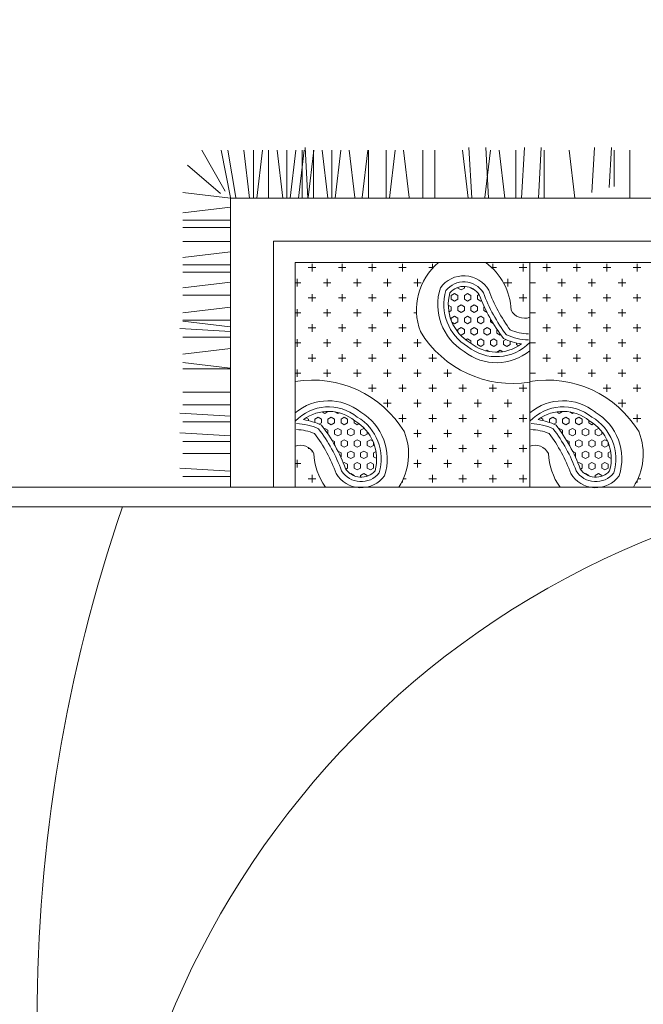
# Model space of a CAD drawing. Units: inches. Extents: x -638 to 186, y -762 to 59.
# Tile 8 of 31: x -140 to -118, y -492 to -457. Entities that reach past the tile are written whole.
import ezdxf

# ---------------------------------------------------------------- set-up
doc = ezdxf.new("R2010")
doc.units = ezdxf.units.IN
doc.layers.add('A-ANNO-DIMS', color=2, linetype='Continuous', lineweight=18)
doc.layers.add('furn', color=8, linetype='Continuous', lineweight=13)
doc.styles.get("Standard").update_dxf_attribs({"font": 'arial.ttf'})
doc.dimstyles.new('ISO-25', dxfattribs={"dimtxt": 4, "dimasz": 4, "dimexe": 1.25, "dimexo": 0.625, "dimtad": 0, "dimlunit": 4, "dimtxsty": 'Standard', "dimcen": 2.5, "dimclrt": 256, "dimadec": 0, "dimazin": 0, "dimtfac": 1, "dimtmove": 0, "dimatfit": 3, "dimfxl": 1, "dimfxlon": 1, "dimarcsym": 0})

# ---------------------------------------------------------------- blocks, each defined once
blk = doc.blocks.new('BED-DOUBLE-WITH-NIGHTSTANDS')
for p, q in [((58.548, 11.244), (58.548, 59.951)), ((57.828, 13.164), (57.828, 58.468)), ((58.923, 31.914), (58.923, 33.642)), ((59.126, 31.914), (59.228, 33.743)), ((59.755, 31.928), (59.755, 33.639)), ((60.193, 31.914), (60.193, 33.642)), ((60.397, 31.914), (60.499, 33.743)), ((60.906, 31.914), (60.906, 33.642)), ((61.11, 31.914), (61.212, 33.743)), ((61.517, 31.914), (61.517, 33.642)), ((61.977, 31.914), (61.977, 33.642)), ((62.81, 31.928), (62.81, 33.639)), ((62.841, 31.928), (63.044, 33.642)), ((63.554, 31.914), (63.35, 33.642)), ((63.961, 31.914), (63.961, 33.642)), ((64.165, 31.914), (64.266, 33.743)), ((64.327, 31.928), (64.531, 33.642)), ((64.572, 31.914), (64.572, 33.642)), ((65.04, 31.914), (64.836, 33.642)), ((65.476, 31.914), (65.476, 33.642)), ((65.944, 31.914), (65.741, 33.642)), ((66.309, 31.928), (66.309, 33.639)), ((66.573, 31.914), (66.573, 33.642)), ((67.041, 31.914), (66.838, 33.642)), ((67.406, 31.928), (67.406, 33.639)), ((67.922, 31.928), (67.922, 33.639)), ((68.186, 31.914), (68.186, 33.642)), ((68.654, 31.914), (68.45, 33.642)), ((68.982, 31.914), (69.186, 33.642)), ((69.142, 32.273), (70.169, 33.468)), ((69.232, 32.112), (70.71, 32.951)), ((68.996, 31.914), (70.707, 32.257)), ((68.996, 31.721), (70.707, 32.011)), ((58.548, 31.914), (68.982, 31.914)), ((68.982, 31.914), (68.982, 1.829)), ((68.982, 31.232), (70.71, 31.436)), ((68.982, 30.966), (70.71, 30.762)), ((68.996, 31.086), (70.707, 31.086)), ((58.548, 30.359), (67.427, 30.359)), ((67.427, 30.359), (67.427, 3.384)), ((68.982, 30.547), (70.71, 30.547)), ((68.982, 30.033), (70.71, 30.237)), ((68.996, 29.887), (70.707, 29.887)), ((58.548, 29.582), (66.65, 29.582)), ((59.258, 29.515), (59.53, 29.515)), ((59.394, 29.379), (59.394, 29.582)), ((62.523, 29.515), (62.795, 29.515)), ((62.659, 29.379), (62.659, 29.582)), ((63.612, 29.515), (63.884, 29.515)), ((63.748, 29.379), (63.748, 29.582)), ((64.7, 29.515), (64.972, 29.515)), ((64.836, 29.379), (64.836, 29.582)), ((65.788, 29.515), (66.06, 29.515)), ((65.924, 29.379), (65.924, 29.582)), ((66.65, 29.582), (66.65, 4.161)), ((68.982, 29.767), (70.71, 29.563)), ((61.047, 29.18), (61.003, 29.104)), ((68.982, 29.46), (70.71, 29.256)), ((68.982, 29.324), (70.71, 29.324)), ((68.982, 29.121), (70.811, 29.223)), ((58.714, 28.971), (58.986, 28.971)), ((58.85, 28.835), (58.85, 29.107)), ((59.802, 28.971), (59.857, 28.971)), ((59.938, 29.054), (59.938, 29.107)), ((61.003, 28.869), (60.881, 28.869)), ((61.003, 29.104), (60.948, 29.104)), ((61.003, 28.869), (61.072, 28.751)), ((63.067, 28.971), (63.339, 28.971)), ((63.203, 28.835), (63.203, 29.107)), ((64.156, 28.971), (64.428, 28.971)), ((64.292, 28.835), (64.292, 29.107)), ((65.244, 28.971), (65.516, 28.971)), ((65.38, 28.835), (65.38, 29.107)), ((66.332, 28.971), (66.605, 28.971)), ((66.468, 28.835), (66.468, 29.107)), ((68.982, 28.917), (70.71, 28.917)), ((68.996, 29.116), (70.71, 28.912)), ((60.663, 28.515), (60.595, 28.397)), ((60.652, 28.534), (60.663, 28.515)), ((60.821, 28.713), (60.867, 28.633)), ((61.003, 28.633), (60.867, 28.633)), ((61.072, 28.751), (61.003, 28.633)), ((61.261, 28.608), (61.208, 28.515)), ((61.208, 28.515), (61.276, 28.397)), ((62.659, 28.291), (62.659, 28.563)), ((63.748, 28.291), (63.748, 28.563)), ((64.836, 28.291), (64.836, 28.563)), ((65.924, 28.291), (65.924, 28.563)), ((68.982, 28.403), (70.71, 28.606)), ((60.187, 28.162), (60.075, 28.162)), ((60.245, 28.262), (60.187, 28.162)), ((60.459, 28.162), (60.391, 28.044)), ((60.459, 28.399), (60.459, 28.397)), ((60.595, 28.397), (60.459, 28.397)), ((60.595, 28.162), (60.459, 28.162)), ((60.595, 28.162), (60.663, 28.044)), ((60.867, 28.397), (60.799, 28.28)), ((60.799, 28.28), (60.867, 28.162)), ((61.003, 28.397), (60.867, 28.397)), ((61.003, 28.162), (60.867, 28.162)), ((61.003, 28.397), (61.072, 28.28)), ((61.072, 28.28), (61.003, 28.162)), ((61.258, 28.131), (61.208, 28.044)), ((61.279, 28.397), (61.276, 28.397)), ((62.523, 28.427), (62.795, 28.427)), ((63.612, 28.427), (63.884, 28.427)), ((64.7, 28.427), (64.972, 28.427)), ((65.788, 28.427), (66.06, 28.427)), ((68.982, 28.136), (70.71, 27.933)), ((68.996, 28.256), (70.707, 28.256)), ((59.199, 27.753), (59.235, 27.69)), ((59.439, 27.808), (59.371, 27.69)), ((59.419, 27.842), (59.439, 27.808)), ((59.637, 27.937), (59.643, 27.926)), ((59.779, 27.926), (59.643, 27.926)), ((59.843, 28.037), (59.779, 27.926)), ((60.051, 27.926), (59.983, 27.808)), ((59.983, 27.808), (60.051, 27.69)), ((60.187, 27.926), (60.051, 27.926)), ((60.187, 27.926), (60.255, 27.808)), ((60.255, 27.808), (60.187, 27.69)), ((60.391, 28.044), (60.459, 27.926)), ((60.595, 27.926), (60.459, 27.926)), ((60.663, 28.044), (60.595, 27.926)), ((60.867, 27.926), (60.799, 27.808)), ((60.799, 27.808), (60.867, 27.69)), ((61.003, 27.926), (60.867, 27.926)), ((61.003, 27.926), (61.072, 27.808)), ((61.072, 27.808), (61.003, 27.69)), ((61.208, 28.044), (61.231, 28.004)), ((63.067, 27.883), (63.339, 27.883)), ((63.203, 27.747), (63.203, 28.019)), ((64.156, 27.883), (64.428, 27.883)), ((64.292, 27.747), (64.292, 28.019)), ((65.244, 27.883), (65.516, 27.883)), ((65.38, 27.747), (65.38, 28.019)), ((66.332, 27.883), (66.605, 27.883)), ((66.468, 27.747), (66.468, 28.019)), ((58.963, 27.455), (58.955, 27.455)), ((59.031, 27.573), (58.963, 27.455)), ((59.025, 27.583), (59.031, 27.573)), ((59.235, 27.455), (59.167, 27.337)), ((59.371, 27.69), (59.235, 27.69)), ((59.371, 27.455), (59.235, 27.455)), ((59.371, 27.455), (59.439, 27.337)), ((59.643, 27.69), (59.575, 27.573)), ((59.575, 27.573), (59.643, 27.455)), ((59.779, 27.69), (59.643, 27.69)), ((59.779, 27.455), (59.643, 27.455)), ((59.779, 27.69), (59.847, 27.573)), ((59.847, 27.573), (59.779, 27.455)), ((60.051, 27.455), (59.983, 27.337)), ((60.187, 27.69), (60.051, 27.69)), ((60.187, 27.455), (60.051, 27.455)), ((60.187, 27.455), (60.255, 27.337)), ((60.459, 27.69), (60.391, 27.573)), ((60.391, 27.573), (60.459, 27.455)), ((60.595, 27.69), (60.459, 27.69)), ((60.595, 27.455), (60.459, 27.455)), ((60.595, 27.69), (60.663, 27.573)), ((60.663, 27.573), (60.595, 27.455)), ((60.867, 27.455), (60.799, 27.337)), ((61.003, 27.69), (60.867, 27.69)), ((60.958, 27.455), (60.867, 27.455)), ((62.659, 27.203), (62.659, 27.475)), ((63.748, 27.203), (63.748, 27.475)), ((64.836, 27.203), (64.836, 27.475)), ((65.924, 27.203), (65.924, 27.475)), ((68.996, 27.424), (70.71, 27.627)), ((58.963, 27.219), (58.904, 27.219)), ((58.963, 27.219), (59.031, 27.101)), ((59.031, 27.101), (58.963, 26.984)), ((59.167, 27.337), (59.235, 27.219)), ((59.371, 27.219), (59.235, 27.219)), ((59.439, 27.337), (59.371, 27.219)), ((59.643, 27.219), (59.575, 27.101)), ((59.575, 27.101), (59.643, 26.984)), ((59.779, 27.219), (59.643, 27.219)), ((59.779, 27.219), (59.847, 27.101)), ((59.847, 27.101), (59.779, 26.984)), ((59.983, 27.337), (60.051, 27.219)), ((60.187, 27.219), (60.051, 27.219)), ((60.255, 27.337), (60.187, 27.219)), ((60.459, 27.219), (60.391, 27.101)), ((60.391, 27.101), (60.459, 26.984)), ((60.595, 27.219), (60.459, 27.219)), ((60.595, 27.219), (60.663, 27.101)), ((60.663, 27.101), (60.637, 27.055)), ((60.799, 27.337), (60.836, 27.274)), ((62.523, 27.339), (62.795, 27.339)), ((63.612, 27.339), (63.884, 27.339)), ((64.7, 27.339), (64.972, 27.339)), ((65.788, 27.339), (66.06, 27.339)), ((68.996, 27.156), (70.71, 26.953)), ((58.963, 26.984), (58.94, 26.984)), ((59.235, 26.984), (59.167, 26.866)), ((59.167, 26.866), (59.235, 26.748)), ((59.371, 26.984), (59.235, 26.984)), ((59.371, 26.748), (59.235, 26.748)), ((59.371, 26.984), (59.439, 26.866)), ((59.439, 26.866), (59.371, 26.748)), ((59.643, 26.748), (59.58, 26.638)), ((59.779, 26.984), (59.643, 26.984)), ((59.779, 26.748), (59.643, 26.748)), ((59.779, 26.748), (59.83, 26.661)), ((60.051, 26.984), (59.983, 26.866)), ((59.983, 26.866), (60.051, 26.748)), ((60.187, 26.984), (60.051, 26.984)), ((60.144, 26.748), (60.051, 26.748)), ((60.187, 26.984), (60.255, 26.866)), ((60.255, 26.866), (60.201, 26.772)), ((60.553, 26.984), (60.459, 26.984)), ((61.979, 26.795), (62.251, 26.795)), ((62.115, 26.659), (62.115, 26.931)), ((63.067, 26.795), (63.339, 26.795)), ((63.203, 26.659), (63.203, 26.931)), ((64.156, 26.795), (64.428, 26.795)), ((64.292, 26.659), (64.292, 26.931)), ((65.244, 26.795), (65.516, 26.795)), ((65.38, 26.659), (65.38, 26.931)), ((66.332, 26.795), (66.605, 26.795)), ((66.468, 26.659), (66.468, 26.931)), ((68.996, 26.933), (70.707, 26.933)), ((61.571, 26.114), (61.571, 26.386)), ((62.659, 26.114), (62.659, 26.386)), ((63.748, 26.114), (63.748, 26.386)), ((64.836, 26.114), (64.836, 26.386)), ((65.924, 26.114), (65.924, 26.386)), ((61.435, 26.25), (61.707, 26.25)), ((62.523, 26.25), (62.795, 26.25)), ((63.612, 26.25), (63.884, 26.25)), ((64.7, 26.25), (64.972, 26.25)), ((65.788, 26.25), (66.06, 26.25)), ((68.982, 26.177), (70.71, 25.974)), ((68.996, 26.297), (70.707, 26.297)), ((58.714, 25.706), (58.783, 25.706)), ((58.85, 25.57), (58.85, 25.675)), ((60.891, 25.706), (61.163, 25.706)), ((61.027, 25.57), (61.027, 25.842)), ((61.979, 25.706), (62.251, 25.706)), ((62.115, 25.57), (62.115, 25.842)), ((63.067, 25.706), (63.339, 25.706)), ((63.203, 25.57), (63.203, 25.842)), ((64.156, 25.706), (64.428, 25.706)), ((64.292, 25.57), (64.292, 25.842)), ((65.244, 25.706), (65.516, 25.706)), ((65.38, 25.57), (65.38, 25.842)), ((66.332, 25.706), (66.605, 25.706)), ((66.468, 25.57), (66.468, 25.842)), ((68.996, 25.465), (70.71, 25.668)), ((59.394, 25.026), (59.394, 25.298)), ((60.483, 25.026), (60.483, 25.298)), ((61.571, 25.026), (61.571, 25.298)), ((62.659, 25.026), (62.659, 25.298)), ((63.748, 25.026), (63.748, 25.298)), ((64.836, 25.2), (64.836, 25.298)), ((65.924, 25.026), (65.924, 25.298)), ((59.258, 25.162), (59.53, 25.162)), ((60.346, 25.162), (60.619, 25.162)), ((61.435, 25.162), (61.707, 25.162)), ((62.523, 25.162), (62.795, 25.162)), ((63.612, 25.162), (63.884, 25.162)), ((65.788, 25.162), (66.06, 25.162)), ((68.996, 24.973), (70.707, 24.973)), ((58.714, 24.618), (58.986, 24.618)), ((58.85, 24.482), (58.85, 24.754)), ((59.802, 24.618), (60.074, 24.618)), ((59.938, 24.482), (59.938, 24.754)), ((60.891, 24.618), (61.163, 24.618)), ((61.027, 24.482), (61.027, 24.754)), ((61.979, 24.618), (62.251, 24.618)), ((62.115, 24.482), (62.115, 24.754)), ((63.067, 24.618), (63.339, 24.618)), ((63.203, 24.482), (63.203, 24.754)), ((66.45, 24.618), (66.605, 24.618)), ((66.468, 24.601), (66.468, 24.754)), ((68.996, 24.543), (70.707, 24.543)), ((59.394, 23.938), (59.394, 24.21)), ((60.483, 23.938), (60.483, 24.21)), ((61.571, 23.938), (61.571, 24.21)), ((62.659, 23.938), (62.659, 24.21)), ((59.258, 24.074), (59.53, 24.074)), ((60.346, 24.074), (60.619, 24.074)), ((61.435, 24.074), (61.707, 24.074)), ((62.523, 24.074), (62.795, 24.074)), ((64.44, 23.825), (64.495, 23.919)), ((64.508, 23.707), (64.44, 23.825)), ((64.552, 23.942), (64.644, 23.942)), ((64.712, 23.825), (64.644, 23.942)), ((64.644, 23.707), (64.712, 23.825)), ((64.917, 23.942), (64.866, 24.03)), ((64.917, 23.942), (65.053, 23.942)), ((65.053, 23.942), (65.116, 24.052)), ((65.257, 23.825), (65.325, 23.942)), ((65.325, 23.707), (65.257, 23.825)), ((65.325, 23.942), (65.461, 23.942)), ((65.529, 23.825), (65.461, 23.942)), ((65.461, 23.707), (65.529, 23.825)), ((58.714, 23.53), (58.986, 23.53)), ((58.85, 23.393), (58.85, 23.666)), ((59.802, 23.53), (60.074, 23.53)), ((59.938, 23.393), (59.938, 23.666)), ((60.891, 23.53), (61.163, 23.53)), ((61.027, 23.393), (61.027, 23.666)), ((61.979, 23.53), (62.251, 23.53)), ((62.115, 23.393), (62.115, 23.666)), ((64.032, 23.589), (64.059, 23.635)), ((64.1, 23.471), (64.032, 23.589)), ((64.1, 23.471), (64.236, 23.471)), ((64.143, 23.707), (64.236, 23.707)), ((64.304, 23.589), (64.236, 23.707)), ((64.236, 23.471), (64.304, 23.589)), ((64.44, 23.353), (64.508, 23.471)), ((64.508, 23.707), (64.644, 23.707)), ((64.508, 23.471), (64.644, 23.471)), ((64.712, 23.353), (64.644, 23.471)), ((64.849, 23.589), (64.917, 23.707)), ((64.917, 23.471), (64.849, 23.589)), ((64.917, 23.707), (65.053, 23.707)), ((64.917, 23.471), (65.053, 23.471)), ((65.121, 23.589), (65.053, 23.707)), ((65.053, 23.471), (65.121, 23.589)), ((65.257, 23.353), (65.325, 23.471)), ((65.325, 23.707), (65.461, 23.707)), ((65.325, 23.471), (65.461, 23.471)), ((65.529, 23.353), (65.461, 23.471)), ((65.665, 23.589), (65.733, 23.707)), ((65.733, 23.471), (65.665, 23.589)), ((65.733, 23.707), (65.755, 23.707)), ((65.733, 23.471), (65.791, 23.471)), ((68.982, 23.339), (70.71, 23.542)), ((59.394, 22.849), (59.394, 23.121)), ((60.483, 22.849), (60.483, 23.121)), ((61.571, 22.849), (61.571, 23.121)), ((63.737, 23.235), (63.828, 23.235)), ((63.828, 23.235), (63.896, 23.353)), ((63.896, 23.353), (63.86, 23.416)), ((64.032, 23.118), (64.1, 23.235)), ((64.1, 23), (64.032, 23.118)), ((64.1, 23.235), (64.236, 23.235)), ((64.304, 23.118), (64.236, 23.235)), ((64.236, 23), (64.304, 23.118)), ((64.508, 23.235), (64.44, 23.353)), ((64.508, 23.235), (64.644, 23.235)), ((64.644, 23.235), (64.712, 23.353)), ((64.849, 23.118), (64.917, 23.235)), ((64.917, 23), (64.849, 23.118)), ((64.917, 23.235), (65.053, 23.235)), ((65.121, 23.118), (65.053, 23.235)), ((65.053, 23), (65.121, 23.118)), ((65.325, 23.235), (65.257, 23.353)), ((65.325, 23.235), (65.461, 23.235)), ((65.461, 23.235), (65.529, 23.353)), ((65.665, 23.118), (65.733, 23.235)), ((65.671, 23.107), (65.665, 23.118)), ((65.733, 23.235), (65.741, 23.235)), ((68.982, 23.207), (70.811, 23.309)), ((59.258, 22.985), (59.53, 22.985)), ((60.346, 22.985), (60.619, 22.985)), ((61.435, 22.985), (61.707, 22.985)), ((63.624, 22.882), (63.692, 23)), ((63.692, 22.764), (63.624, 22.882)), ((63.692, 23), (63.828, 23)), ((63.692, 22.764), (63.828, 22.764)), ((63.896, 22.882), (63.828, 23)), ((63.828, 22.764), (63.896, 22.882)), ((64.032, 22.646), (64.1, 22.764)), ((64.1, 23), (64.236, 23)), ((64.1, 22.764), (64.236, 22.764)), ((64.304, 22.646), (64.236, 22.764)), ((64.44, 22.882), (64.508, 23)), ((64.508, 22.764), (64.44, 22.882)), ((64.508, 23), (64.644, 23)), ((64.508, 22.764), (64.644, 22.764)), ((64.712, 22.882), (64.644, 23)), ((64.644, 22.764), (64.712, 22.882)), ((64.852, 22.653), (64.917, 22.764)), ((64.917, 23), (65.053, 23)), ((64.917, 22.764), (65.053, 22.764)), ((65.059, 22.753), (65.053, 22.764)), ((65.257, 22.882), (65.325, 23)), ((65.276, 22.848), (65.257, 22.882)), ((65.325, 23), (65.461, 23)), ((65.497, 22.937), (65.461, 23)), ((58.714, 22.441), (58.986, 22.441)), ((58.85, 22.305), (58.85, 22.577)), ((59.802, 22.441), (60.074, 22.441)), ((59.938, 22.305), (59.938, 22.577)), ((60.891, 22.441), (61.163, 22.441)), ((61.027, 22.305), (61.027, 22.577)), ((61.979, 22.441), (62.251, 22.441)), ((62.115, 22.305), (62.115, 22.577)), ((63.438, 22.559), (63.488, 22.646)), ((63.488, 22.646), (63.465, 22.686)), ((63.624, 22.411), (63.692, 22.529)), ((63.692, 22.293), (63.624, 22.411)), ((63.692, 22.529), (63.828, 22.529)), ((63.896, 22.411), (63.828, 22.529)), ((63.828, 22.293), (63.896, 22.411)), ((64.1, 22.529), (64.032, 22.646)), ((64.1, 22.529), (64.236, 22.529)), ((64.236, 22.529), (64.304, 22.646)), ((64.451, 22.428), (64.508, 22.529)), ((64.508, 22.529), (64.621, 22.529)), ((66.43, 22.441), (66.605, 22.441)), ((66.468, 22.305), (66.468, 22.481)), ((68.982, 22.596), (70.811, 22.698)), ((68.996, 22.728), (70.71, 22.524)), ((63.417, 22.293), (63.42, 22.293)), ((63.488, 22.175), (63.42, 22.293)), ((63.434, 22.082), (63.488, 22.175)), ((63.624, 21.939), (63.692, 22.057)), ((63.692, 22.293), (63.828, 22.293)), ((63.692, 22.057), (63.828, 22.057)), ((63.874, 21.977), (63.828, 22.057)), ((64.032, 22.175), (64.1, 22.293)), ((64.043, 22.156), (64.032, 22.175)), ((64.1, 22.293), (64.236, 22.293)), ((64.237, 22.292), (64.236, 22.293)), ((68.982, 22.015), (70.71, 22.219)), ((59.258, 21.897), (59.53, 21.897)), ((59.394, 21.761), (59.394, 22.033)), ((60.346, 21.897), (60.619, 21.897)), ((60.483, 21.761), (60.483, 22.033)), ((61.435, 21.897), (61.707, 21.897)), ((61.571, 21.761), (61.571, 22.033)), ((63.692, 21.822), (63.624, 21.939)), ((63.692, 21.822), (63.815, 21.822)), ((65.788, 21.897), (66.06, 21.897)), ((65.924, 21.761), (65.924, 22.033)), ((58.714, 21.353), (58.986, 21.353)), ((58.85, 21.217), (58.85, 21.489)), ((59.802, 21.353), (60.074, 21.353)), ((59.938, 21.217), (59.938, 21.489)), ((60.891, 21.353), (61.163, 21.353)), ((61.027, 21.217), (61.027, 21.489)), ((61.979, 21.353), (62.251, 21.353)), ((62.115, 21.217), (62.115, 21.489)), ((63.648, 21.51), (63.692, 21.586)), ((63.692, 21.586), (63.748, 21.586)), ((65.244, 21.353), (65.516, 21.353)), ((65.38, 21.217), (65.38, 21.489)), ((66.332, 21.353), (66.605, 21.353)), ((66.468, 21.217), (66.468, 21.489)), ((68.982, 21.608), (70.71, 21.608)), ((68.982, 21.404), (70.811, 21.302)), ((58.548, 21.108), (66.65, 21.108)), ((62.659, 20.906), (62.659, 21.108)), ((63.748, 20.906), (63.748, 21.108)), ((64.836, 20.906), (64.836, 21.108)), ((65.924, 20.906), (65.924, 21.108)), ((61.003, 20.631), (60.948, 20.631)), ((61.047, 20.707), (61.003, 20.631)), ((63.203, 20.362), (63.203, 20.634)), ((64.292, 20.362), (64.292, 20.634)), ((65.38, 20.362), (65.38, 20.634)), ((66.468, 20.362), (66.468, 20.634)), ((68.982, 20.793), (70.811, 20.691)), ((61.003, 20.395), (60.881, 20.395)), ((61.003, 20.395), (61.072, 20.277)), ((61.072, 20.277), (61.003, 20.159)), ((63.067, 20.498), (63.339, 20.498)), ((64.156, 20.498), (64.428, 20.498)), ((65.244, 20.498), (65.516, 20.498)), ((66.332, 20.498), (66.605, 20.498)), ((68.982, 20.59), (70.71, 20.59)), ((60.459, 19.925), (60.459, 19.924)), ((60.595, 19.924), (60.459, 19.924)), ((60.663, 20.042), (60.595, 19.924)), ((60.652, 20.061), (60.663, 20.042)), ((60.867, 19.924), (60.799, 19.806)), ((60.821, 20.239), (60.867, 20.159)), ((61.003, 20.159), (60.867, 20.159)), ((61.003, 19.924), (60.867, 19.924)), ((61.003, 19.924), (61.072, 19.806)), ((61.261, 20.135), (61.208, 20.042)), ((61.208, 20.042), (61.276, 19.924)), ((61.279, 19.924), (61.276, 19.924)), ((62.523, 19.954), (62.795, 19.954)), ((62.659, 19.817), (62.659, 20.09)), ((63.612, 19.954), (63.884, 19.954)), ((63.748, 19.817), (63.748, 20.09)), ((64.7, 19.954), (64.972, 19.954)), ((64.836, 19.817), (64.836, 20.09)), ((65.788, 19.954), (66.06, 19.954)), ((65.924, 19.817), (65.924, 20.09)), ((59.843, 19.564), (59.779, 19.453)), ((60.187, 19.688), (60.075, 19.688)), ((60.245, 19.788), (60.187, 19.688)), ((60.459, 19.688), (60.391, 19.57)), ((60.391, 19.57), (60.459, 19.453)), ((60.595, 19.688), (60.459, 19.688)), ((60.595, 19.688), (60.663, 19.57)), ((60.663, 19.57), (60.595, 19.453)), ((60.799, 19.806), (60.867, 19.688)), ((61.003, 19.688), (60.867, 19.688)), ((61.072, 19.806), (61.003, 19.688)), ((61.258, 19.657), (61.208, 19.57)), ((61.208, 19.57), (61.231, 19.53)), ((68.982, 19.485), (70.71, 19.689)), ((59.199, 19.28), (59.235, 19.217)), ((59.371, 19.217), (59.235, 19.217)), ((59.439, 19.335), (59.371, 19.217)), ((59.419, 19.369), (59.439, 19.335)), ((59.643, 19.217), (59.575, 19.099)), ((59.637, 19.464), (59.643, 19.453)), ((59.779, 19.453), (59.643, 19.453)), ((59.779, 19.217), (59.643, 19.217)), ((59.779, 19.217), (59.847, 19.099)), ((60.051, 19.453), (59.983, 19.335)), ((59.983, 19.335), (60.051, 19.217)), ((60.187, 19.453), (60.051, 19.453)), ((60.187, 19.217), (60.051, 19.217)), ((60.187, 19.453), (60.255, 19.335)), ((60.255, 19.335), (60.187, 19.217)), ((60.459, 19.217), (60.391, 19.099)), ((60.595, 19.453), (60.459, 19.453)), ((60.595, 19.217), (60.459, 19.217)), ((60.595, 19.217), (60.663, 19.099)), ((60.867, 19.453), (60.799, 19.335)), ((60.799, 19.335), (60.867, 19.217)), ((61.003, 19.453), (60.867, 19.453)), ((61.003, 19.217), (60.867, 19.217)), ((61.003, 19.453), (61.072, 19.335)), ((61.072, 19.335), (61.003, 19.217)), ((63.067, 19.409), (63.339, 19.409)), ((63.203, 19.273), (63.203, 19.545)), ((64.156, 19.409), (64.428, 19.409)), ((64.292, 19.273), (64.292, 19.545)), ((65.244, 19.409), (65.516, 19.409)), ((65.38, 19.273), (65.38, 19.545)), ((66.332, 19.409), (66.605, 19.409)), ((66.468, 19.273), (66.468, 19.545)), ((58.963, 18.981), (58.955, 18.981)), ((59.031, 19.099), (58.963, 18.981)), ((59.025, 19.109), (59.031, 19.099)), ((59.235, 18.981), (59.167, 18.863)), ((59.167, 18.863), (59.235, 18.746)), ((59.371, 18.981), (59.235, 18.981)), ((59.371, 18.981), (59.439, 18.863)), ((59.439, 18.863), (59.371, 18.746)), ((59.575, 19.099), (59.643, 18.981)), ((59.779, 18.981), (59.643, 18.981)), ((59.847, 19.099), (59.779, 18.981)), ((60.051, 18.981), (59.983, 18.863)), ((59.983, 18.863), (60.051, 18.746)), ((60.187, 18.981), (60.051, 18.981)), ((60.187, 18.981), (60.255, 18.863)), ((60.255, 18.863), (60.187, 18.746)), ((60.391, 19.099), (60.459, 18.981)), ((60.595, 18.981), (60.459, 18.981)), ((60.663, 19.099), (60.595, 18.981)), ((60.867, 18.981), (60.799, 18.863)), ((60.799, 18.863), (60.836, 18.801)), ((60.958, 18.981), (60.867, 18.981)), ((62.523, 18.865), (62.795, 18.865)), ((62.659, 18.729), (62.659, 19.001)), ((63.612, 18.865), (63.884, 18.865)), ((63.748, 18.729), (63.748, 19.001)), ((64.7, 18.865), (64.972, 18.865)), ((64.836, 18.729), (64.836, 19.001)), ((65.788, 18.865), (66.06, 18.865)), ((65.924, 18.729), (65.924, 19.001)), ((69.184, 18.863), (70.811, 18.772)), ((58.963, 18.746), (58.904, 18.746)), ((58.963, 18.51), (58.94, 18.51)), ((58.963, 18.746), (59.031, 18.628)), ((59.031, 18.628), (58.963, 18.51)), ((59.235, 18.51), (59.167, 18.392)), ((59.371, 18.746), (59.235, 18.746)), ((59.371, 18.51), (59.235, 18.51)), ((59.371, 18.51), (59.439, 18.392)), ((59.643, 18.746), (59.575, 18.628)), ((59.575, 18.628), (59.643, 18.51)), ((59.779, 18.746), (59.643, 18.746)), ((59.779, 18.51), (59.643, 18.51)), ((59.779, 18.746), (59.847, 18.628)), ((59.847, 18.628), (59.779, 18.51)), ((60.051, 18.51), (59.983, 18.392)), ((60.187, 18.746), (60.051, 18.746)), ((60.187, 18.51), (60.051, 18.51)), ((60.187, 18.51), (60.255, 18.392)), ((60.459, 18.746), (60.391, 18.628)), ((60.391, 18.628), (60.459, 18.51)), ((60.595, 18.746), (60.459, 18.746)), ((60.553, 18.51), (60.459, 18.51)), ((60.595, 18.746), (60.663, 18.628)), ((60.663, 18.628), (60.637, 18.582)), ((59.167, 18.392), (59.235, 18.274)), ((59.371, 18.274), (59.235, 18.274)), ((59.439, 18.392), (59.371, 18.274)), ((59.643, 18.274), (59.58, 18.165)), ((59.779, 18.274), (59.643, 18.274)), ((59.779, 18.274), (59.83, 18.187)), ((59.983, 18.392), (60.051, 18.274)), ((60.144, 18.274), (60.051, 18.274)), ((60.255, 18.392), (60.201, 18.298)), ((61.979, 18.321), (62.251, 18.321)), ((62.115, 18.185), (62.115, 18.457)), ((63.067, 18.321), (63.339, 18.321)), ((63.203, 18.185), (63.203, 18.457)), ((64.156, 18.321), (64.428, 18.321)), ((64.292, 18.185), (64.292, 18.457)), ((65.244, 18.321), (65.516, 18.321)), ((65.38, 18.185), (65.38, 18.457)), ((66.332, 18.321), (66.605, 18.321)), ((66.468, 18.185), (66.468, 18.457)), ((69.357, 18.243), (70.811, 18.162)), ((61.435, 17.777), (61.707, 17.777)), ((61.571, 17.641), (61.571, 17.913)), ((62.523, 17.777), (62.795, 17.777)), ((62.659, 17.641), (62.659, 17.913)), ((63.612, 17.777), (63.884, 17.777)), ((63.748, 17.641), (63.748, 17.913)), ((64.7, 17.777), (64.972, 17.777)), ((64.836, 17.641), (64.836, 17.913)), ((65.788, 17.777), (66.06, 17.777)), ((65.924, 17.641), (65.924, 17.913)), ((69.393, 18.06), (70.71, 18.06)), ((68.982, 17.492), (70.707, 17.492)), ((58.714, 17.233), (58.783, 17.233)), ((58.85, 17.097), (58.85, 17.202)), ((60.891, 17.233), (61.163, 17.233)), ((61.027, 17.097), (61.027, 17.369)), ((61.979, 17.233), (62.251, 17.233)), ((62.115, 17.097), (62.115, 17.369)), ((63.067, 17.233), (63.339, 17.233)), ((63.203, 17.097), (63.203, 17.369)), ((64.156, 17.233), (64.428, 17.233)), ((64.292, 17.097), (64.292, 17.369)), ((65.244, 17.233), (65.516, 17.233)), ((65.38, 17.097), (65.38, 17.369)), ((66.332, 17.233), (66.605, 17.233)), ((66.468, 17.097), (66.468, 17.369))]:
    blk.add_line(p, q)
for centre, radius, start, end in [((39.353, -18.016), 56.914, 71.0577, 108.9423), ((27.358, 4.824), 31.662, 15.7708, 101.8099), ((59.514, 29.388), 0.54, 297.0088, 21.0409), ((58.736, 29.604), 1.887, 337.4091, 358.0373), ((58.53, 28.957), 3.88, 301.1125, 9.2666), ((58.736, 29.604), 2.104, 335.7609, 358.0373), ((59.782, 28.381), 1.66, 321.1107, 46.3387), ((59.782, 28.381), 1.878, 321.5973, 39.7611), ((58.736, 29.604), 2.268, 334.7059, 351.7535), ((59.782, 28.381), 1.497, 320.6541, 36.833), ((59.856, 26.664), 2.246, 92.4675, 125.6302), ((57.143, 33.342), 5.571, 289.9219, 306.7677), ((57.143, 33.342), 5.789, 290.1318, 307.346), ((57.143, 33.342), 5.952, 290.2997, 307.7385), ((59.57, 27.2), 1.047, 120.344, 234.0192), ((59.57, 27.2), 0.829, 121.6232, 231.6957), ((59.57, 27.2), 0.666, 122.9498, 229.099), ((59.563, 28.229), 1.591, 254.3738, 329.9117), ((59.563, 28.229), 1.972, 252.055, 329.019), ((59.563, 28.229), 1.754, 253.2189, 329.4808), ((59.74, 27.689), 2.202, 237.1993, 291.1583), ((66.165, 21.733), 3.88, 121.1125, 189.2666), ((64.955, 23.002), 2.202, 39.6653, 111.1583), ((65.133, 22.461), 1.972, 72.055, 149.019), ((65.133, 22.461), 1.754, 73.2189, 149.4808), ((65.126, 23.49), 1.047, 300.344, 54.0192), ((65.133, 22.461), 1.591, 74.3738, 149.9117), ((65.126, 23.49), 0.666, 302.9498, 49.099), ((65.126, 23.49), 0.829, 301.6232, 51.6957), ((64.914, 22.31), 1.878, 141.5973, 219.7611), ((64.914, 22.31), 1.66, 141.1107, 226.3387), ((64.914, 22.31), 1.497, 140.6541, 216.833), ((67.553, 17.348), 5.952, 110.2997, 127.7385), ((67.553, 17.348), 5.789, 110.1318, 127.346), ((67.553, 17.348), 5.571, 109.9219, 126.7677), ((64.84, 24.027), 2.246, 272.4675, 323.7193), ((65.96, 21.087), 2.268, 154.7059, 171.7535), ((65.96, 21.087), 2.104, 155.7609, 178.0373), ((65.96, 21.087), 1.887, 157.4091, 178.0373), ((65.181, 21.302), 0.54, 117.0088, 201.0409), ((59.514, 20.915), 0.54, 297.0088, 21.0409), ((58.736, 21.13), 1.887, 337.4091, 358.0373), ((58.53, 20.484), 3.88, 301.1125, 9.2666), ((58.736, 21.13), 2.104, 335.7609, 358.0373), ((59.782, 19.907), 1.66, 321.1107, 46.3387), ((59.782, 19.907), 1.878, 321.5973, 39.7611), ((58.736, 21.13), 2.268, 334.7059, 351.7535), ((59.782, 19.907), 1.497, 320.6541, 36.833), ((59.856, 18.19), 2.246, 92.4675, 125.6302), ((57.143, 24.868), 5.571, 289.9219, 306.7677), ((57.143, 24.868), 5.789, 290.1318, 307.346), ((57.143, 24.868), 5.952, 290.2997, 307.7385), ((59.57, 18.727), 1.047, 120.344, 234.0192), ((59.57, 18.727), 0.829, 121.6232, 231.6957), ((59.57, 18.727), 0.666, 122.9498, 229.099), ((59.563, 19.756), 1.754, 253.2189, 329.4808), ((59.563, 19.756), 1.591, 254.3738, 329.9117), ((59.563, 19.756), 1.972, 252.055, 329.019), ((59.74, 19.215), 2.202, 237.1993, 291.1583)]:
    blk.add_arc(centre, radius, start, end)
blk = doc.blocks.new('*D38')
at = {"layer": 'A-ANNO-DIMS', "color": 0, "lineweight": -2, "transparency": 16777216}
for p, q in [((182.663, -280.533), (184.913, -280.533)), ((183.663, -284.533), (183.663, -371.726)), ((183.663, -473.533), (183.663, -386.34)), ((182.663, -477.533), (184.913, -477.533))]:
    blk.add_line(p, q, dxfattribs=at)
at = {"layer": 'A-ANNO-DIMS', "color": 0, "lineweight": 30, "transparency": 16777216}
for points in [[(182.997, -284.533), (184.33, -284.533), (183.663, -280.533)], [(182.997, -473.533), (184.33, -473.533), (183.663, -477.533)]]:
    blk.add_solid(points, dxfattribs=at)
at = {"layer": 'Defpoints', "color": 0, "lineweight": 30, "transparency": 16777216}
for p in [(-404.526, -280.533), (-404.526, -477.533), (183.663, -477.533)]:
    blk.add_point(p, dxfattribs=at)
at = {"layer": 'A-ANNO-DIMS', "transparency": 16777216, "insert": (183.663, -379.033), "char_height": 4, "attachment_point": 5, "rotation": 90}
blk.add_mtext('16\'-5"', dxfattribs=at)

msp = doc.modelspace()

# ---------------------------------------------------------------- block references
at = {"layer": 'furn', "rotation": 90.00000000000017}
msp.add_blockref('BED-DOUBLE-WITH-NIGHTSTANDS', (-100.575, -532.203), dxfattribs=at)

# ---------------------------------------------------------------- dimensions: what is measured, and where the dimension line sits
at = {"layer": 'A-ANNO-DIMS'}
dim = msp.add_linear_dim(base=(183.663, -477.533), p1=(-404.526, -280.533), p2=(-404.526, -477.533), angle=90, dimstyle='ISO-25', override={"dimdec": 1, "dimlfac": 1, "dimrnd": 0, "dimzin": 1, "dimdsep": 46, "dimlunit": 4, "dimfrac": 2}, dxfattribs=at)
dim.commit()
dim.dimension.update_dxf_attribs({"geometry": '*D38', "text_midpoint": (183.663, -379.033)})

doc.saveas('drawing.dxf')
